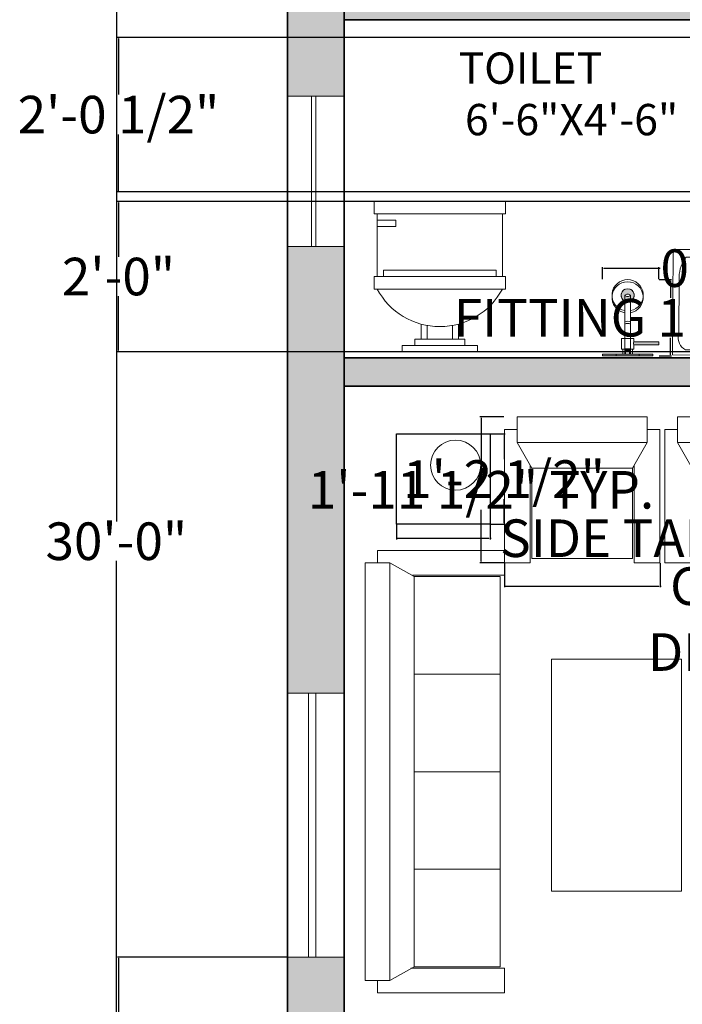
# Model space of a CAD drawing. Units: inches. Extents: x 143233372 to 143233714, y 112671713 to 112672292.
# Tile 2 of 7: x 143233373 to 143233479, y 112671935 to 112672092. Entities that reach past the tile are written whole.
import ezdxf

# ---------------------------------------------------------------- set-up
doc = ezdxf.new("R2010")
doc.units = ezdxf.units.IN
doc.header["$MEASUREMENT"] = 0
doc.layers.get('0').update_dxf_attribs({"color": 104})
for name, color, linetype, lineweight in [('A-ANNO-DIMS', 2, 'Continuous', 18), ('A-AREA-IDEN', 7, 'Continuous', 18), ('furniture', 23, 'Continuous', 18), ('PLUMBING FIXTURES', 8, 'Continuous', 18), ('walls', 7, 'Continuous', 35), ('windows', 4, 'Continuous', 18)]:
    doc.layers.add(name, color=color, linetype=linetype, lineweight=lineweight)
doc.layers.add('A-WALL-PATT', color=18, linetype='Continuous', lineweight=9, true_color=0x000000)
doc.layers.add('table', color=140, linetype='Continuous')
doc.styles.get("Standard").update_dxf_attribs({"font": 'arial.ttf'})
doc.dimstyles.get("Standard").update_dxf_attribs({"dimtxt": 6, "dimasz": 0.18, "dimexe": 0.18, "dimexo": 0.0625, "dimgap": 0.09, "dimtad": 0, "dimtih": 1, "dimtoh": 1, "dimzin": 0, "dimdsep": 46, "dimlunit": 3, "dimtxsty": 'Standard', "dimcen": 0.09, "dimadec": 0, "dimazin": 0, "dimtfac": 1, "dimtofl": 0, "dimtmove": 0, "dimatfit": 3, "dimfxl": 1, "dimtolj": 1, "dimtzin": 0, "dimarcsym": 0})

# ---------------------------------------------------------------- blocks, each defined once
blk = doc.blocks.new('FABRIC SOFA 4S')
at = {"layer": 'furniture'}
for p, q in [((3, 54), (34, 54)), ((3, 51), (3, 54)), ((34, 48), (34, 54)), ((0, -51), (0, 51)), ((6, 51), (0, 51)), ((6, -51), (6, 51)), ((12, 47.63), (6, 51)), ((11.14, 48), (34, 48)), ((33, 23.81), (12, 23.81)), ((33, 0), (12, 0)), ((33, -23.81), (12, -23.81)), ((6, -51), (12, -47.63)), ((11.54, -48), (34, -48)), ((34, -48), (34, -54)), ((6, -51), (0, -51)), ((3, -54), (3, -51)), ((3, -54), (34, -54))]:
    blk.add_line(p, q, dxfattribs=at)
blk.add_lwpolyline([(12, -47.63), (12, 47.63), (33, 47.63), (33, -47.63)], close=True, dxfattribs=at)
blk = doc.blocks.new('table')
at = {"layer": 'furniture'}
blk.add_circle((2425.82, 1326.97), 6.64, dxfattribs=at)
at = {"layer": 'table'}
blk.add_line((2410.17, 1335.23), (2434.94, 1335.23), dxfattribs=at)
blk = doc.blocks.new('support table')
at = {"layer": 'table'}
for p, q in [((-15.66, -15.62), (-15.66, 8.26)), ((9.12, 8.26), (9.12, -15.62)), ((9.12, -15.62), (-15.66, -15.62))]:
    blk.add_line(p, q, dxfattribs=at)
at = {"layer": 'furniture'}
blk.add_blockref('table', (-2425.82, -1326.97), dxfattribs=at)
blk = doc.blocks.new('FABRIC SOFA 1S')
at = {"layer": 'furniture'}
for p, q in [((3, 18.12), (34, 18.12)), ((3, 15.12), (3, 18.12)), ((34, 12.12), (34, 18.12)), ((0, -15.12), (0, 15.12)), ((6, 15.12), (0, 15.12)), ((6, -15.12), (6, 15.12)), ((12, 11.75), (6, 15.12)), ((11.33, 12.12), (34, 12.12)), ((6, -15.12), (12, -11.75)), ((11.33, -12.12), (34, -12.12)), ((34, -12.12), (34, -18.12)), ((6, -15.12), (0, -15.12)), ((3, -18.12), (3, -15.12)), ((3, -18.12), (34, -18.12))]:
    blk.add_line(p, q, dxfattribs=at)
blk.add_lwpolyline([(12, -11.75), (12, 11.75), (33, 11.75), (33, -11.75)], close=True, dxfattribs=at)
blk = doc.blocks.new('*U19')
for p, q in [((-10, 22), (-10, 12)), ((-10, 21), (-7, 21)), ((-7, 21), (-7, 20)), ((10, 12), (10, 22)), ((-7, 20), (-10, 20)), ((9, 13), (-9, 13)), ((-9, 13), (-9, 12)), ((9, 12), (9, 13)), ((10.5, 12), (-10.5, 12)), ((-10.5, 10), (-10.5, 12)), ((10.5, 12), (10.5, 10)), ((10.5, 10), (-10.5, 10)), ((-3, 4.4065), (-3, 2)), ((-2, 2), (-2, 4.1658)), ((2, 4.1658), (2, 2)), ((3, 2), (3, 4.4065)), ((4, 2), (-4, 2)), ((-4, 2), (-4, 1)), ((4, 1), (4, 2))]:
    blk.add_line(p, q)
for points in [[(10.5, 22), (10.5, 24), (-10.5, 24), (-10.5, 22)], [(6, 0), (6, 1), (-6, 1), (-6, 0)]]:
    blk.add_lwpolyline(points, close=True)
blk.add_arc((0, 15.3333), 11.3333, 208.0725, 331.9275)
blk = doc.blocks.new('O.H SHOWER-PL')
at = {"layer": 'PLUMBING FIXTURES'}
for points in [[(-1.84, 0), (-1.84, -0.25), (1.84, -0.25), (1.84, 0)], [(0.46, -8.72), (0.46, -9.67, -0.422337), (-0.46, -9.67), (-0.46, -8.72, 4.325472)]]:
    blk.add_hatch(color=256, dxfattribs=at).paths.add_polyline_path(points)
for p, q in [((-1.84, 0), (-1.84, -0.25)), ((1.84, 0), (-1.84, 0)), ((1.84, 0), (1.84, -0.25)), ((1.84, -0.25), (-1.84, -0.25)), ((-0.46, -0.25), (-0.46, -9.67)), ((0.46, -0.25), (0.46, -9.67))]:
    blk.add_line(p, q, dxfattribs=at)
for centre, radius, start, end in [((0, -4.48), 1.03, 243.53, 296.47), ((0, -9.67), 2.5, 100.61, 79.39), ((0, -9.67), 1.05, 116.0349, 63.9652), ((0, -9.22), 0.643, 224.2078, 315.7922)]:
    blk.add_arc(centre, radius, start, end, dxfattribs=at)
blk = doc.blocks.new('DIVERTER-PL')
at = {"layer": 'PLUMBING FIXTURES'}
for points in [[(4, 0), (-4, 0), (-4, -0.25), (4, -0.25)], [(0.38, -1.14), (0.38, -0.7), (-0.37, -0.7), (-0.37, -1.14)], [(1, -1.75, 0.30818), (1, -2.25), (5, -2.25), (5, -1.75)]]:
    blk.add_hatch(color=256, dxfattribs=at).paths.add_polyline_path(points)
for p, q in [((-4, 0), (-4, -0.25)), ((-4, 0), (4, 0)), ((4, 0), (4, -0.25)), ((-4, -0.25), (4, -0.25)), ((-4, -0.25), (4, -0.25)), ((-1, -1.05), (-0.37, -1.05)), ((-1, -1.05), (-1, -2.75)), ((-0.75, -0.25), (-0.75, -1.05)), ((-0.37, -0.7), (0.38, -0.7)), ((-0.37, -0.7), (-0.37, -1.14)), ((-0.37, -1.14), (0.38, -1.14)), ((-0.32, -0.7), (-0.32, -0.25)), ((0.32, -0.7), (0.32, -0.25)), ((0.38, -0.7), (0.38, -1.14)), ((0.38, -1.05), (1, -1.05)), ((0.75, -0.25), (0.75, -1.05)), ((1, -1.05), (1, -1.75)), ((-1, -2.75), (1, -2.75)), ((1, -2.25), (1, -2.75))]:
    blk.add_line(p, q, dxfattribs=at)
at = {"layer": 'PLUMBING FIXTURES', "ltscale": 12}
for p, q in [((1, -1.75), (5, -1.75)), ((1, -2.25), (5, -2.25)), ((5, -2.25), (5, -1.75))]:
    blk.add_line(p, q, dxfattribs=at)
at = {"layer": 'PLUMBING FIXTURES'}
blk.add_arc((1.37, -2), 0.444, 145.7435, 214.2565, dxfattribs=at)
blk = doc.blocks.new('A$C7F153053')
at = {"layer": 'PLUMBING FIXTURES', "xscale": -1, "rotation": 270}
for name in ['DIVERTER-PL', 'O.H SHOWER-PL']:
    blk.add_blockref(name, (12.17, 4), dxfattribs=at)
blk = doc.blocks.new('*D28')
at = {"layer": 'A-ANNO-DIMS', "color": 0, "lineweight": -2, "transparency": 16777216}
for p, q in [((143233416.22, 112672249.18), (143233388.75, 112672249.18)), ((143233388.93, 112672249), (143233388.93, 112672011.59)), ((143233388.93, 112671767.86), (143233388.93, 112672005.28)), ((143233416.22, 112671767.68), (143233388.75, 112671767.68))]:
    blk.add_line(p, q, dxfattribs=at)
at = {"layer": 'A-ANNO-DIMS', "color": 0, "transparency": 16777216}
for points in [[(143233388.9, 112672249), (143233388.96, 112672249), (143233388.93, 112672249.18)], [(143233388.9, 112671767.86), (143233388.96, 112671767.86), (143233388.93, 112671767.68)]]:
    blk.add_solid(points, dxfattribs=at)
at = {"layer": 'Defpoints', "color": 0, "transparency": 16777216}
for p in [(143233416.28, 112672249.18), (143233388.93, 112671767.68), (143233416.28, 112671767.68)]:
    blk.add_point(p, dxfattribs=at)
at = {"layer": 'A-ANNO-DIMS', "color": 0, "transparency": 16777216, "insert": (143233388.93, 112672008.43), "char_height": 6, "attachment_point": 5}
blk.add_mtext('\\A1;30\'-0"', dxfattribs=at)
blk = doc.blocks.new('SASH-42IN')
for p, q in [((0, 1.17), (42.12, 1.17)), ((42.12, 0), (0, 0)), ((42.12, 1.17), (42.12, 0))]:
    blk.add_line(p, q)
blk = doc.blocks.new('LAVATORY-RECT')
for p, q in [((0, 0.15), (0.11, 17)), ((0.11, 17), (23.11, 16.85)), ((20.97, 15.65), (2.15, 15.77)), ((23.11, 16.85), (23.1, 15.71)), ((23.1, 15.71), (23, 0)), ((0.99, 3.35), (1.05, 12.64)), ((21.96, 3.21), (22.03, 12.5)), ((11.22, 9.73), (11.16, 9.24)), ((11.36, 9.22), (11.4, 9.7)), ((10.4, 8.91), (9.84, 8.81)), ((10.52, 8.7), (9.87, 8.58)), ((11.84, 8.39), (12.22, 7.95)), ((11.97, 8.6), (12.36, 8.13)), ((23, 0), (0, 0.15)), ((21.95, 0.84), (2.06, 0.97))]:
    blk.add_line(p, q)
for radius in [2.61, 1.39, 0.816, 0.338]:
    blk.add_circle((11.22, 8.91), radius)
for centre, radius, start, end in [((6.46, 12.5), 5.4, 142.7525, 178.5493), ((16.62, 12.43), 5.4, 0.6949, 36.4918), ((3, 2.82), 2.08, 165.2338, 242.9258), ((12.7, 2.09), 9.33, 352.3124, 6.9318)]:
    blk.add_arc(centre, radius, start, end)
blk = doc.blocks.new('SHOWER-ARM-AND-HEAD')
blk.add_hatch(color=256).paths.add_polyline_path([(2.05, 10.36), (2.05, 9.42, 0.422337), (2.97, 9.42), (2.97, 10.36, -4.325472)])
blk.add_hatch(color=256).paths.add_polyline_path([(2.05, 10.36), (2.05, 9.42, 0.422337), (2.97, 9.42), (2.97, 10.36, -4.325472)])
blk.add_hatch(color=256).paths.add_polyline_path([(2.05, 10.36), (2.05, 9.42, 0.422337), (2.97, 9.42), (2.97, 10.36, -4.325472)])
blk.add_hatch(color=256).paths.add_polyline_path([(2.05, 10.36), (2.05, 9.42, 0.422337), (2.97, 9.42), (2.97, 10.36, -4.325472)])
blk.add_hatch(color=256).paths.add_polyline_path([(2.05, 10.36), (2.05, 9.42, 0.422337), (2.97, 9.42), (2.97, 10.36, -4.325472)])
blk.add_hatch(color=256).paths.add_polyline_path([(2.05, 10.36), (2.05, 9.42, 0.422337), (2.97, 9.42), (2.97, 10.36, -4.325472)])
blk.add_hatch(color=256).paths.add_polyline_path([(2.05, 10.36), (2.05, 9.42, 0.422337), (2.97, 9.42), (2.97, 10.36, -4.325472)])
blk.add_hatch(color=256).paths.add_polyline_path([(2.05, 10.36), (2.05, 9.42, 0.422337), (2.97, 9.42), (2.97, 10.36, -4.325472)])
blk.add_hatch(color=256).paths.add_polyline_path([(2.05, 10.36), (2.05, 9.42, 0.422337), (2.97, 9.42), (2.97, 10.36, -4.325472)])
blk.add_hatch(color=256).paths.add_polyline_path([(2.05, 10.36), (2.05, 9.42, 0.422337), (2.97, 9.42), (2.97, 10.36, -4.325472)])
blk.add_hatch(color=256).paths.add_polyline_path([(2.05, 10.36), (2.05, 9.42, 0.422337), (2.97, 9.42), (2.97, 10.36, -4.325472)])
blk.add_hatch(color=256).paths.add_polyline_path([(2.05, 10.36), (2.05, 9.42, 0.422337), (2.97, 9.42), (2.97, 10.36, -4.325472)])
blk.add_hatch(color=256).paths.add_polyline_path([(2.05, 10.36), (2.05, 9.42, 0.422337), (2.97, 9.42), (2.97, 10.36, -4.325472)])
blk.add_hatch(color=256).paths.add_polyline_path([(2.05, 10.36), (2.05, 9.42, 0.422337), (2.97, 9.42), (2.97, 10.36, -4.325472)])
blk.add_hatch(color=256).paths.add_polyline_path([(2.05, 10.36), (2.05, 9.42, 0.422337), (2.97, 9.42), (2.97, 10.36, -4.325472)])
blk.add_hatch(color=256).paths.add_polyline_path([(2.05, 10.36), (2.05, 9.42, 0.422337), (2.97, 9.42), (2.97, 10.36, -4.325472)])
blk.add_hatch(color=256).paths.add_polyline_path([(2.05, 10.36), (2.05, 9.42, 0.422337), (2.97, 9.42), (2.97, 10.36, -4.325472)])
blk.add_hatch(color=256).paths.add_polyline_path([(2.05, 10.36), (2.05, 9.42, 0.422337), (2.97, 9.42), (2.97, 10.36, -4.325472)])
blk.add_hatch(color=256).paths.add_polyline_path([(2.05, 10.36), (2.05, 9.42, 0.422337), (2.97, 9.42), (2.97, 10.36, -4.325472)])
blk.add_hatch(color=256).paths.add_polyline_path([(2.05, 10.36), (2.05, 9.42, 0.422337), (2.97, 9.42), (2.97, 10.36, -4.325472)])
blk.add_hatch(color=256).paths.add_polyline_path([(2.05, 10.36), (2.05, 9.42, 0.422337), (2.97, 9.42), (2.97, 10.36, -4.325472)])
blk.add_hatch(color=256).paths.add_polyline_path([(2.05, 10.36), (2.05, 9.42, 0.422337), (2.97, 9.42), (2.97, 10.36, -4.325472)])
blk.add_hatch(color=256).paths.add_polyline_path([(2.05, 10.36), (2.05, 9.42, 0.422337), (2.97, 9.42), (2.97, 10.36, -4.325472)])
blk.add_hatch(color=256).paths.add_polyline_path([(2.05, 10.36), (2.05, 9.42, 0.422337), (2.97, 9.42), (2.97, 10.36, -4.325472)])
blk.add_hatch(color=256).paths.add_polyline_path([(2.05, 10.36), (2.05, 9.42, 0.422337), (2.97, 9.42), (2.97, 10.36, -4.325472)])
blk.add_hatch(color=256).paths.add_polyline_path([(2.05, 10.36), (2.05, 9.42, 0.422337), (2.97, 9.42), (2.97, 10.36, -4.325472)])
blk.add_hatch(color=256).paths.add_polyline_path([(2.05, 10.36), (2.05, 9.42, 0.422337), (2.97, 9.42), (2.97, 10.36, -4.325472)])
blk.add_hatch(color=256).paths.add_polyline_path([(2.05, 10.36), (2.05, 9.42, 0.422337), (2.97, 9.42), (2.97, 10.36, -4.325472)])
blk.add_hatch(color=256).paths.add_polyline_path([(2.05, 10.36), (2.05, 9.42, 0.422337), (2.97, 9.42), (2.97, 10.36, -4.325472)])
blk.add_hatch(color=256).paths.add_polyline_path([(2.05, 10.36), (2.05, 9.42, 0.422337), (2.97, 9.42), (2.97, 10.36, -4.325472)])
blk.add_hatch(color=256).paths.add_polyline_path([(2.05, 10.36), (2.05, 9.42, 0.422337), (2.97, 9.42), (2.97, 10.36, -4.325472)])
blk.add_hatch(color=256).paths.add_polyline_path([(2.05, 10.36), (2.05, 9.42, 0.422337), (2.97, 9.42), (2.97, 10.36, -4.325472)])
blk.add_hatch(color=256).paths.add_polyline_path([(2.05, 10.36), (2.05, 9.42, 0.422337), (2.97, 9.42), (2.97, 10.36, -4.325472)])
blk.add_hatch(color=256).paths.add_polyline_path([(2.05, 10.36), (2.05, 9.42, 0.422337), (2.97, 9.42), (2.97, 10.36, -4.325472)])
blk.add_hatch(color=256).paths.add_polyline_path([(2.05, 10.36), (2.05, 9.42, 0.422337), (2.97, 9.42), (2.97, 10.36, -4.325472)])
blk.add_hatch(color=256).paths.add_polyline_path([(2.05, 10.36), (2.05, 9.42, 0.422337), (2.97, 9.42), (2.97, 10.36, -4.325472)])
blk.add_hatch(color=256).paths.add_polyline_path([(2.05, 10.36), (2.05, 9.42, 0.422337), (2.97, 9.42), (2.97, 10.36, -4.325472)])
blk.add_hatch(color=256).paths.add_polyline_path([(2.05, 10.36), (2.05, 9.42, 0.422337), (2.97, 9.42), (2.97, 10.36, -4.325472)])
for p, q in [((2.05, 0), (2.05, 9.42)), ((2.05, 0), (2.05, 9.42)), ((2.05, 0), (2.05, 9.42)), ((2.05, 0), (2.05, 9.42)), ((2.05, 0), (2.05, 9.42)), ((2.05, 0), (2.05, 9.42)), ((2.05, 0), (2.05, 9.42)), ((2.05, 0), (2.05, 9.42)), ((2.05, 0), (2.05, 9.42)), ((2.05, 0), (2.05, 9.42)), ((2.05, 0), (2.05, 9.42)), ((2.05, 0), (2.05, 9.42)), ((2.05, 0), (2.05, 9.42)), ((2.05, 0), (2.05, 9.42)), ((2.05, 0), (2.05, 9.42)), ((2.05, 0), (2.05, 9.42)), ((2.05, 0), (2.05, 9.42)), ((2.05, 0), (2.05, 9.42)), ((2.05, 0), (2.05, 9.42)), ((2.05, 0), (2.05, 9.42)), ((2.05, 0), (2.05, 9.42)), ((2.05, 0), (2.05, 9.42)), ((2.05, 0), (2.05, 9.42)), ((2.05, 0), (2.05, 9.42)), ((2.05, 0), (2.05, 9.42)), ((2.05, 0), (2.05, 9.42)), ((2.05, 0), (2.05, 9.42)), ((2.05, 0), (2.05, 9.42)), ((2.05, 0), (2.05, 9.42)), ((2.05, 0), (2.05, 9.42)), ((2.05, 0), (2.05, 9.42)), ((2.05, 0), (2.05, 9.42)), ((2.05, 0), (2.05, 9.42)), ((2.05, 0), (2.05, 9.42)), ((2.05, 0), (2.05, 9.42)), ((2.05, 0), (2.05, 9.42)), ((2.05, 0), (2.05, 9.42)), ((2.05, 0), (2.05, 9.42)), ((2.97, 0), (2.97, 9.42)), ((2.97, 0), (2.97, 9.42)), ((2.97, 0), (2.97, 9.42)), ((2.97, 0), (2.97, 9.42)), ((2.97, 0), (2.97, 9.42)), ((2.97, 0), (2.97, 9.42)), ((2.97, 0), (2.97, 9.42)), ((2.97, 0), (2.97, 9.42)), ((2.97, 0), (2.97, 9.42)), ((2.97, 0), (2.97, 9.42)), ((2.97, 0), (2.97, 9.42)), ((2.97, 0), (2.97, 9.42)), ((2.97, 0), (2.97, 9.42)), ((2.97, 0), (2.97, 9.42)), ((2.97, 0), (2.97, 9.42)), ((2.97, 0), (2.97, 9.42)), ((2.97, 0), (2.97, 9.42)), ((2.97, 0), (2.97, 9.42)), ((2.97, 0), (2.97, 9.42)), ((2.97, 0), (2.97, 9.42)), ((2.97, 0), (2.97, 9.42)), ((2.97, 0), (2.97, 9.42)), ((2.97, 0), (2.97, 9.42)), ((2.97, 0), (2.97, 9.42)), ((2.97, 0), (2.97, 9.42)), ((2.97, 0), (2.97, 9.42)), ((2.97, 0), (2.97, 9.42)), ((2.97, 0), (2.97, 9.42)), ((2.97, 0), (2.97, 9.42)), ((2.97, 0), (2.97, 9.42)), ((2.97, 0), (2.97, 9.42)), ((2.97, 0), (2.97, 9.42)), ((2.97, 0), (2.97, 9.42)), ((2.97, 0), (2.97, 9.42)), ((2.97, 0), (2.97, 9.42)), ((2.97, 0), (2.97, 9.42)), ((2.97, 0), (2.97, 9.42)), ((2.97, 0), (2.97, 9.42))]:
    blk.add_line(p, q)
for centre, radius, start, end in [((2.5, 9.07), 2.5, 280.61, 259.39), ((2.5, 9.07), 2.5, 280.61, 259.39), ((2.5, 9.07), 2.5, 280.61, 259.39), ((2.5, 9.07), 2.5, 280.61, 259.39), ((2.5, 9.07), 2.5, 280.61, 259.39), ((2.5, 9.07), 2.5, 280.61, 259.39), ((2.5, 9.07), 2.5, 280.61, 259.39), ((2.5, 9.07), 2.5, 280.61, 259.39), ((2.5, 9.07), 2.5, 280.61, 259.39), ((2.5, 9.07), 2.5, 280.61, 259.39), ((2.5, 9.07), 2.5, 280.61, 259.39), ((2.5, 9.07), 2.5, 280.61, 259.39), ((2.5, 9.07), 2.5, 280.61, 259.39), ((2.5, 9.07), 2.5, 280.61, 259.39), ((2.5, 9.07), 2.5, 280.61, 259.39), ((2.5, 9.07), 2.5, 280.61, 259.39), ((2.5, 9.07), 2.5, 280.61, 259.39), ((2.5, 9.07), 2.5, 280.61, 259.39), ((2.5, 9.07), 2.5, 280.61, 259.39), ((2.5, 9.07), 2.5, 280.61, 259.39), ((2.5, 9.07), 2.5, 280.61, 259.39), ((2.5, 9.07), 2.5, 280.61, 259.39), ((2.5, 9.07), 2.5, 280.61, 259.39), ((2.5, 9.07), 2.5, 280.61, 259.39), ((2.5, 9.07), 2.5, 280.61, 259.39), ((2.5, 9.07), 2.5, 280.61, 259.39), ((2.5, 9.07), 2.5, 280.61, 259.39), ((2.5, 9.07), 2.5, 280.61, 259.39), ((2.5, 9.07), 2.5, 280.61, 259.39), ((2.5, 9.07), 2.5, 280.61, 259.39), ((2.5, 9.07), 2.5, 280.61, 259.39), ((2.5, 9.07), 2.5, 280.61, 259.39), ((2.5, 9.07), 2.5, 280.61, 259.39), ((2.5, 9.07), 2.5, 280.61, 259.39), ((2.5, 9.07), 2.5, 280.61, 259.39), ((2.5, 9.07), 2.5, 280.61, 259.39), ((2.5, 9.07), 2.5, 280.61, 259.39), ((2.5, 9.07), 2.5, 280.61, 259.39), ((2.51, 9.42), 1.05, 116.0348, 63.9651), ((2.51, 9.42), 1.05, 116.0348, 63.9651), ((2.51, 9.42), 1.05, 116.0348, 63.9651), ((2.51, 9.42), 1.05, 116.0348, 63.9651), ((2.51, 9.42), 1.05, 116.0348, 63.9651), ((2.51, 9.42), 1.05, 116.0348, 63.9651), ((2.51, 9.42), 1.05, 116.0348, 63.9651), ((2.51, 9.42), 1.05, 116.0348, 63.9651), ((2.51, 9.42), 1.05, 116.0348, 63.9651), ((2.51, 9.42), 1.05, 116.0348, 63.9651), ((2.51, 9.42), 1.05, 116.0348, 63.9651), ((2.51, 9.42), 1.05, 116.0348, 63.9651), ((2.51, 9.42), 1.05, 116.0348, 63.9651), ((2.51, 9.42), 1.05, 116.0348, 63.9651), ((2.51, 9.42), 1.05, 116.0348, 63.9651), ((2.51, 9.42), 1.05, 116.0348, 63.9651), ((2.51, 9.42), 1.05, 116.0348, 63.9651), ((2.51, 9.42), 1.05, 116.0348, 63.9651), ((2.51, 9.42), 1.05, 116.0348, 63.9651), ((2.51, 9.42), 1.05, 116.0348, 63.9651), ((2.51, 9.42), 1.05, 116.0348, 63.9651), ((2.51, 9.42), 1.05, 116.0348, 63.9651), ((2.51, 9.42), 1.05, 116.0348, 63.9651), ((2.51, 9.42), 1.05, 116.0348, 63.9651), ((2.51, 9.42), 1.05, 116.0348, 63.9651), ((2.51, 9.42), 1.05, 116.0348, 63.9651), ((2.51, 9.42), 1.05, 116.0348, 63.9651), ((2.51, 9.42), 1.05, 116.0348, 63.9651), ((2.51, 9.42), 1.05, 116.0348, 63.9651), ((2.51, 9.42), 1.05, 116.0348, 63.9651), ((2.51, 9.42), 1.05, 116.0348, 63.9651), ((2.51, 9.42), 1.05, 116.0348, 63.9651), ((2.51, 9.42), 1.05, 116.0348, 63.9651), ((2.51, 9.42), 1.05, 116.0348, 63.9651), ((2.51, 9.42), 1.05, 116.0348, 63.9651), ((2.51, 9.42), 1.05, 116.0348, 63.9651), ((2.51, 9.42), 1.05, 116.0348, 63.9651), ((2.51, 9.42), 1.05, 116.0348, 63.9651), ((2.51, 9.87), 0.643, 224.2078, 315.7922), ((2.51, 9.87), 0.643, 224.2078, 315.7922), ((2.51, 9.87), 0.643, 224.2078, 315.7922), ((2.51, 9.87), 0.643, 224.2078, 315.7922), ((2.51, 9.87), 0.643, 224.2078, 315.7922), ((2.51, 9.87), 0.643, 224.2078, 315.7922), ((2.51, 9.87), 0.643, 224.2078, 315.7922), ((2.51, 9.87), 0.643, 224.2078, 315.7922), ((2.51, 9.87), 0.643, 224.2078, 315.7922), ((2.51, 9.87), 0.643, 224.2078, 315.7922), ((2.51, 9.87), 0.643, 224.2078, 315.7922), ((2.51, 9.87), 0.643, 224.2078, 315.7922), ((2.51, 9.87), 0.643, 224.2078, 315.7922), ((2.51, 9.87), 0.643, 224.2078, 315.7922), ((2.51, 9.87), 0.643, 224.2078, 315.7922), ((2.51, 9.87), 0.643, 224.2078, 315.7922), ((2.51, 9.87), 0.643, 224.2078, 315.7922), ((2.51, 9.87), 0.643, 224.2078, 315.7922), ((2.51, 9.87), 0.643, 224.2078, 315.7922), ((2.51, 9.87), 0.643, 224.2078, 315.7922), ((2.51, 9.87), 0.643, 224.2078, 315.7922), ((2.51, 9.87), 0.643, 224.2078, 315.7922), ((2.51, 9.87), 0.643, 224.2078, 315.7922), ((2.51, 9.87), 0.643, 224.2078, 315.7922), ((2.51, 9.87), 0.643, 224.2078, 315.7922), ((2.51, 9.87), 0.643, 224.2078, 315.7922), ((2.51, 9.87), 0.643, 224.2078, 315.7922), ((2.51, 9.87), 0.643, 224.2078, 315.7922), ((2.51, 9.87), 0.643, 224.2078, 315.7922), ((2.51, 9.87), 0.643, 224.2078, 315.7922), ((2.51, 9.87), 0.643, 224.2078, 315.7922), ((2.51, 9.87), 0.643, 224.2078, 315.7922), ((2.51, 9.87), 0.643, 224.2078, 315.7922), ((2.51, 9.87), 0.643, 224.2078, 315.7922), ((2.51, 9.87), 0.643, 224.2078, 315.7922), ((2.51, 9.87), 0.643, 224.2078, 315.7922), ((2.51, 9.87), 0.643, 224.2078, 315.7922), ((2.51, 9.87), 0.643, 224.2078, 315.7922), ((2.5, 3.88), 1.03, 63.53, 116.47), ((2.5, 3.88), 1.03, 63.53, 116.47), ((2.5, 3.88), 1.03, 63.53, 116.47), ((2.5, 3.88), 1.03, 63.53, 116.47), ((2.5, 3.88), 1.03, 63.53, 116.47), ((2.5, 3.88), 1.03, 63.53, 116.47), ((2.5, 3.88), 1.03, 63.53, 116.47), ((2.5, 3.88), 1.03, 63.53, 116.47), ((2.5, 3.88), 1.03, 63.53, 116.47), ((2.5, 3.88), 1.03, 63.53, 116.47), ((2.5, 3.88), 1.03, 63.53, 116.47), ((2.5, 3.88), 1.03, 63.53, 116.47), ((2.5, 3.88), 1.03, 63.53, 116.47), ((2.5, 3.88), 1.03, 63.53, 116.47), ((2.5, 3.88), 1.03, 63.53, 116.47), ((2.5, 3.88), 1.03, 63.53, 116.47), ((2.5, 3.88), 1.03, 63.53, 116.47), ((2.5, 3.88), 1.03, 63.53, 116.47), ((2.5, 3.88), 1.03, 63.53, 116.47), ((2.5, 3.88), 1.03, 63.53, 116.47), ((2.5, 3.88), 1.03, 63.53, 116.47), ((2.5, 3.88), 1.03, 63.53, 116.47), ((2.5, 3.88), 1.03, 63.53, 116.47), ((2.5, 3.88), 1.03, 63.53, 116.47), ((2.5, 3.88), 1.03, 63.53, 116.47), ((2.5, 3.88), 1.03, 63.53, 116.47), ((2.5, 3.88), 1.03, 63.53, 116.47), ((2.5, 3.88), 1.03, 63.53, 116.47), ((2.5, 3.88), 1.03, 63.53, 116.47), ((2.5, 3.88), 1.03, 63.53, 116.47), ((2.5, 3.88), 1.03, 63.53, 116.47), ((2.5, 3.88), 1.03, 63.53, 116.47), ((2.5, 3.88), 1.03, 63.53, 116.47), ((2.5, 3.88), 1.03, 63.53, 116.47), ((2.5, 3.88), 1.03, 63.53, 116.47), ((2.5, 3.88), 1.03, 63.53, 116.47), ((2.5, 3.88), 1.03, 63.53, 116.47), ((2.5, 3.88), 1.03, 63.53, 116.47)]:
    blk.add_arc(centre, radius, start, end)
blk = doc.blocks.new('*D35')
at = {"layer": 'A-ANNO-DIMS', "color": 0, "lineweight": -2, "transparency": 16777216}
for p, q in [((143233450.89, 112672004.93), (143233450.89, 112672001.08)), ((143233475.74, 112672004.93), (143233475.74, 112672001.08)), ((143233451.07, 112672001.26), (143233475.56, 112672001.26)), ((143233475.74, 112672001.26), (143233475.92, 112672001.26))]:
    blk.add_line(p, q, dxfattribs=at)
at = {"layer": 'A-ANNO-DIMS', "color": 0, "transparency": 16777216}
for points in [[(143233451.07, 112672001.29), (143233451.07, 112672001.23), (143233450.89, 112672001.26)], [(143233475.56, 112672001.29), (143233475.56, 112672001.23), (143233475.74, 112672001.26)]]:
    blk.add_solid(points, dxfattribs=at)
at = {"layer": 'Defpoints', "color": 0, "transparency": 16777216}
for p in [(143233450.89, 112672004.99), (143233475.74, 112672004.99), (143233475.74, 112672001.26)]:
    blk.add_point(p, dxfattribs=at)
at = {"layer": 'A-ANNO-DIMS', "color": 0, "transparency": 16777216, "insert": (143233508.46, 112672001.26), "char_height": 6, "attachment_point": 5}
blk.add_mtext('\\A1;CHAIR 2\'-1" TYP.', dxfattribs=at)
blk = doc.blocks.new('*D36')
at = {"layer": 'A-ANNO-DIMS', "color": 0, "lineweight": -2, "transparency": 16777216}
for p, q in [((143233450.82, 112672028.3), (143233446.98, 112672028.3)), ((143233447.16, 112672028.12), (143233447.16, 112672019.84)), ((143233447.16, 112672005.17), (143233447.16, 112672013.45)), ((143233450.82, 112672004.99), (143233446.98, 112672004.99))]:
    blk.add_line(p, q, dxfattribs=at)
at = {"layer": 'A-ANNO-DIMS', "color": 0, "transparency": 16777216}
for points in [[(143233447.13, 112672028.12), (143233447.19, 112672028.12), (143233447.16, 112672028.3)], [(143233447.13, 112672005.17), (143233447.19, 112672005.17), (143233447.16, 112672004.99)]]:
    blk.add_solid(points, dxfattribs=at)
at = {"layer": 'Defpoints', "color": 0, "transparency": 16777216}
for p in [(143233450.89, 112672028.3), (143233447.16, 112672004.99), (143233450.89, 112672004.99)]:
    blk.add_point(p, dxfattribs=at)
at = {"layer": 'A-ANNO-DIMS', "color": 0, "transparency": 16777216, "insert": (143233447.16, 112672016.64), "char_height": 6, "attachment_point": 5}
blk.add_mtext('\\A1;1\'-11 1/2" TYP.', dxfattribs=at)
blk = doc.blocks.new('*D49')
at = {"layer": 'A-ANNO-DIMS', "color": 0, "lineweight": -2, "transparency": 16777216}
for p, q in [((143233475.63, 112672050.2), (143233477.58, 112672050.2)), ((143233477.4, 112672050.02), (143233477.4, 112672047.31)), ((143233477.4, 112672038.21), (143233477.4, 112672040.92)), ((143233475.63, 112672038.03), (143233477.58, 112672038.03))]:
    blk.add_line(p, q, dxfattribs=at)
at = {"layer": 'A-ANNO-DIMS', "color": 0, "transparency": 16777216}
for points in [[(143233477.37, 112672050.02), (143233477.43, 112672050.02), (143233477.4, 112672050.2)], [(143233477.37, 112672038.21), (143233477.43, 112672038.21), (143233477.4, 112672038.03)]]:
    blk.add_solid(points, dxfattribs=at)
at = {"layer": 'Defpoints', "color": 0, "transparency": 16777216}
for p in [(143233475.57, 112672050.2), (143233475.57, 112672038.03), (143233477.4, 112672038.03)]:
    blk.add_point(p, dxfattribs=at)
at = {"layer": 'A-ANNO-DIMS', "color": 0, "transparency": 16777216, "insert": (143233477.4, 112672044.11), "char_height": 6, "attachment_point": 5}
blk.add_mtext('\\A1;FITTING 1\'-0" TYP.', dxfattribs=at)
blk = doc.blocks.new('*D50')
at = {"layer": 'A-ANNO-DIMS', "color": 0, "lineweight": -2, "transparency": 16777216}
for p, q in [((143233466.57, 112672050.26), (143233466.57, 112672052.2)), ((143233466.75, 112672052.02), (143233475.39, 112672052.02)), ((143233475.57, 112672050.26), (143233475.57, 112672052.2)), ((143233475.57, 112672052.02), (143233475.75, 112672052.02))]:
    blk.add_line(p, q, dxfattribs=at)
at = {"layer": 'A-ANNO-DIMS', "color": 0, "transparency": 16777216}
for points in [[(143233466.75, 112672052.05), (143233466.75, 112672051.99), (143233466.57, 112672052.02)], [(143233475.39, 112672052.05), (143233475.39, 112672051.99), (143233475.57, 112672052.02)]]:
    blk.add_solid(points, dxfattribs=at)
at = {"layer": 'Defpoints', "color": 0, "transparency": 16777216}
for p in [(143233475.57, 112672052.02), (143233466.57, 112672050.2), (143233475.57, 112672050.2)]:
    blk.add_point(p, dxfattribs=at)
at = {"layer": 'A-ANNO-DIMS', "color": 0, "transparency": 16777216, "insert": (143233494.13, 112672052.02), "char_height": 6, "attachment_point": 5}
blk.add_mtext('\\A1;0\'-9" TYP.', dxfattribs=at)
blk = doc.blocks.new('*D55')
at = {"layer": 'A-ANNO-DIMS', "color": 0, "lineweight": -2, "transparency": 16777216}
for p, q in [((143233433.65, 112672011.09), (143233433.65, 112672008.73)), ((143233448.6, 112672011.09), (143233448.6, 112672008.73)), ((143233433.83, 112672008.91), (143233448.42, 112672008.91)), ((143233448.6, 112672008.91), (143233448.78, 112672008.91))]:
    blk.add_line(p, q, dxfattribs=at)
at = {"layer": 'A-ANNO-DIMS', "color": 0, "transparency": 16777216}
for points in [[(143233433.83, 112672008.94), (143233433.83, 112672008.88), (143233433.65, 112672008.91)], [(143233448.42, 112672008.94), (143233448.42, 112672008.88), (143233448.6, 112672008.91)]]:
    blk.add_solid(points, dxfattribs=at)
at = {"layer": 'Defpoints', "color": 0, "transparency": 16777216}
for p in [(143233433.65, 112672011.15), (143233448.6, 112672011.15), (143233448.6, 112672008.91)]:
    blk.add_point(p, dxfattribs=at)
at = {"layer": 'A-ANNO-DIMS', "color": 0, "transparency": 16777216, "insert": (143233482.22, 112672008.91), "char_height": 6, "attachment_point": 5}
blk.add_mtext('\\A1;SIDE TABLE 1\'-3"', dxfattribs=at)
blk = doc.blocks.new('*D56')
at = {"layer": 'A-ANNO-DIMS', "color": 0, "lineweight": -2, "transparency": 16777216}
for p, q in [((143233448.66, 112672025.56), (143233451.02, 112672025.56)), ((143233450.84, 112672025.38), (143233450.84, 112672021.55)), ((143233450.84, 112672011.33), (143233450.84, 112672015.16)), ((143233448.66, 112672011.15), (143233451.02, 112672011.15))]:
    blk.add_line(p, q, dxfattribs=at)
at = {"layer": 'A-ANNO-DIMS', "color": 0, "transparency": 16777216}
for points in [[(143233450.81, 112672025.38), (143233450.87, 112672025.38), (143233450.84, 112672025.56)], [(143233450.81, 112672011.33), (143233450.87, 112672011.33), (143233450.84, 112672011.15)]]:
    blk.add_solid(points, dxfattribs=at)
at = {"layer": 'Defpoints', "color": 0, "transparency": 16777216}
for p in [(143233448.6, 112672025.56), (143233450.84, 112672025.56), (143233448.6, 112672011.15)]:
    blk.add_point(p, dxfattribs=at)
at = {"layer": 'A-ANNO-DIMS', "color": 0, "transparency": 16777216, "insert": (143233450.84, 112672018.35), "char_height": 6, "attachment_point": 5}
blk.add_mtext('\\A1;1\'-2 1/2"', dxfattribs=at)
blk = doc.blocks.new('*D61')
at = {"layer": 'A-ANNO-DIMS', "color": 0, "lineweight": -2, "transparency": 16777216}
for p, q in [((143233522.04, 112672021.05), (143233512.83, 112672021.05)), ((143233513.01, 112672020.87), (143233513.01, 112671993.94)), ((143233513.01, 112671960.62), (143233513.01, 112671987.55)), ((143233522.04, 112671960.44), (143233512.83, 112671960.44))]:
    blk.add_line(p, q, dxfattribs=at)
at = {"layer": 'A-ANNO-DIMS', "color": 0, "transparency": 16777216}
for points in [[(143233512.98, 112672020.87), (143233513.04, 112672020.87), (143233513.01, 112672021.05)], [(143233512.98, 112671960.62), (143233513.04, 112671960.62), (143233513.01, 112671960.44)]]:
    blk.add_solid(points, dxfattribs=at)
at = {"layer": 'Defpoints', "color": 0, "transparency": 16777216}
for p in [(143233513.01, 112672021.05), (143233522.1, 112672021.05), (143233522.1, 112671960.44)]:
    blk.add_point(p, dxfattribs=at)
at = {"layer": 'A-ANNO-DIMS', "color": 0, "transparency": 16777216, "insert": (143233513.01, 112671990.74), "char_height": 6, "attachment_point": 5}
blk.add_mtext('\\A1;DINING SET 5\'-0 1/2"', dxfattribs=at)
blk = doc.blocks.new('*D70')
at = {"layer": 'A-ANNO-DIMS', "color": 0, "lineweight": -2, "transparency": 16777216}
for p, q in [((143233574.42, 112672088.85), (143233389.09, 112672088.85)), ((143233389.27, 112672088.67), (143233389.27, 112672079.72)), ((143233389.27, 112672064.38), (143233389.27, 112672073.33)), ((143233575.22, 112672064.2), (143233389.09, 112672064.2))]:
    blk.add_line(p, q, dxfattribs=at)
at = {"layer": 'A-ANNO-DIMS', "color": 0, "transparency": 16777216}
for points in [[(143233389.24, 112672088.67), (143233389.3, 112672088.67), (143233389.27, 112672088.85)], [(143233389.24, 112672064.38), (143233389.3, 112672064.38), (143233389.27, 112672064.2)]]:
    blk.add_solid(points, dxfattribs=at)
at = {"layer": 'Defpoints', "color": 0, "transparency": 16777216}
for p in [(143233574.48, 112672088.85), (143233389.27, 112672064.2), (143233575.28, 112672064.2)]:
    blk.add_point(p, dxfattribs=at)
at = {"layer": 'A-ANNO-DIMS', "color": 0, "transparency": 16777216, "insert": (143233389.27, 112672076.53), "char_height": 6, "attachment_point": 5}
blk.add_mtext('\\A1;2\'-0 1/2"', dxfattribs=at)
blk = doc.blocks.new('*D72')
at = {"layer": 'A-ANNO-DIMS', "color": 0, "lineweight": -2, "transparency": 16777216}
for p, q in [((143233576.46, 112672062.68), (143233389.09, 112672062.68)), ((143233389.27, 112672062.5), (143233389.27, 112672053.84)), ((143233389.27, 112672038.86), (143233389.27, 112672047.53)), ((143233586.96, 112672038.68), (143233389.09, 112672038.68))]:
    blk.add_line(p, q, dxfattribs=at)
at = {"layer": 'A-ANNO-DIMS', "color": 0, "transparency": 16777216}
for points in [[(143233389.24, 112672062.5), (143233389.3, 112672062.5), (143233389.27, 112672062.68)], [(143233389.24, 112672038.86), (143233389.3, 112672038.86), (143233389.27, 112672038.68)]]:
    blk.add_solid(points, dxfattribs=at)
at = {"layer": 'Defpoints', "color": 0, "transparency": 16777216}
for p in [(143233576.53, 112672062.68), (143233389.27, 112672038.68), (143233587.03, 112672038.68)]:
    blk.add_point(p, dxfattribs=at)
at = {"layer": 'A-ANNO-DIMS', "color": 0, "transparency": 16777216, "insert": (143233389.27, 112672050.68), "char_height": 6, "attachment_point": 5}
blk.add_mtext('\\A1;2\'-0"', dxfattribs=at)
blk = doc.blocks.new('*D73')
at = {"layer": 'A-ANNO-DIMS', "color": 0, "lineweight": -2, "transparency": 16777216}
for p, q in [((143233416.22, 112671942.04), (143233389.09, 112671942.04)), ((143233389.27, 112671941.86), (143233389.27, 112671905.44)), ((143233389.27, 112671862.63), (143233389.27, 112671899.05)), ((143233416.22, 112671862.45), (143233389.09, 112671862.45))]:
    blk.add_line(p, q, dxfattribs=at)
at = {"layer": 'A-ANNO-DIMS', "color": 0, "transparency": 16777216}
for points in [[(143233389.24, 112671941.86), (143233389.3, 112671941.86), (143233389.27, 112671942.04)], [(143233389.24, 112671862.63), (143233389.3, 112671862.63), (143233389.27, 112671862.45)]]:
    blk.add_solid(points, dxfattribs=at)
at = {"layer": 'Defpoints', "color": 0, "transparency": 16777216}
for p in [(143233389.27, 112671942.04), (143233416.28, 112671942.04), (143233416.28, 112671862.45)]:
    blk.add_point(p, dxfattribs=at)
at = {"layer": 'A-ANNO-DIMS', "color": 0, "transparency": 16777216, "insert": (143233389.27, 112671902.24), "char_height": 6, "attachment_point": 5}
blk.add_mtext('\\A1;6\'-7 1/2"', dxfattribs=at)

msp = doc.modelspace()

# ---------------------------------------------------------------- hatches: boundary and pattern name
at = {"layer": 'A-WALL-PATT'}
h = msp.add_hatch(color=256, dxfattribs=at)
h.dxf.hatch_style = 1
h.paths.add_polyline_path([(143233425.285, 112671820.328), (143233416.222, 112671820.328), (143233416.222, 112671767.682), (143233464.805, 112671767.682), (143233464.805, 112671776.682), (143233425.285, 112671776.682)])
h.paths.add_polyline_path([(143233425.285, 112672055.48), (143233416.285, 112672055.48), (143233416.285, 112671984.159), (143233425.285, 112671984.159)])
h.paths.add_polyline_path([(143233656.285, 112671963.912), (143233647.285, 112671963.912), (143233647.285, 112671848.682), (143233647.285, 112671839.682), (143233656.285, 112671839.682), (143233656.285, 112671889.182)])
h.paths.add_polyline_path([(143233425.285, 112672097.332), (143233425.285, 112672097.332), (143233425.285, 112672108.216), (143233425.285, 112672240.182), (143233451.497, 112672240.182), (143233451.497, 112672249.182), (143233416.285, 112672249.182), (143233416.285, 112672079.453), (143233420.069, 112672079.453), (143233425.285, 112672079.453)])
h.paths.add_polyline_path([(143233576.214, 112672249.182), (143233493.616, 112672249.182), (143233493.616, 112672240.182), (143233576.214, 112672240.182)])
h.paths.add_polyline_path([(143233425.285, 112671942.039), (143233416.285, 112671942.039), (143233416.285, 112671889.182), (143233416.271, 112671862.447), (143233425.285, 112671862.447), (143233425.285, 112671896.682), (143233518.63, 112671896.682, -0.0122006), (143233518.603, 112671897.787), (143233518.603, 112671901.182), (143233425.285, 112671901.182)])
h = msp.add_hatch(color=256, dxfattribs=at)
h.dxf.hatch_style = 1
h.paths.add_polyline_path([(143233507.785, 112672062.229), (143233504.087, 112672062.229, -0.0081431), (143233503.285, 112672062.242), (143233503.285, 112672037.682), (143233425.285, 112672037.682), (143233425.285, 112672033.182), (143233507.785, 112672033.182)])
h.paths.add_polyline_path([(143233511.719, 112672096.182), (143233425.285, 112672096.182), (143233425.285, 112672091.682), (143233503.285, 112672091.682), (143233503.285, 112672086.878), (143233504.087, 112672086.878), (143233507.785, 112672086.878), (143233507.785, 112672091.682), (143233511.719, 112672091.682)])

# ---------------------------------------------------------------- linework, layer by layer
at = {"layer": 'furniture'}
for p, q in [((143233433.654, 112672025.56), (143233433.654, 112672011.149)), ((143233448.599, 112672025.56), (143233433.654, 112672025.56)), ((143233448.599, 112672011.149), (143233448.599, 112672025.56)), ((143233433.654, 112672011.149), (143233448.599, 112672011.149)), ((143233458.405, 112671989.621), (143233458.405, 112671952.591)), ((143233479.165, 112671989.621), (143233458.405, 112671989.621)), ((143233479.165, 112671952.591), (143233479.165, 112671989.621)), ((143233458.405, 112671952.591), (143233479.165, 112671952.591))]:
    msp.add_line(p, q, dxfattribs=at)
at = {"layer": 'walls'}
for p, q in [((143233416.285, 112671889.182), (143233416.285, 112672249.182)), ((143233425.285, 112671901.182), (143233425.285, 112672240.182)), ((143233425.285, 112672091.682), (143233503.285, 112672091.682)), ((143233425.285, 112672037.682), (143233503.285, 112672037.682)), ((143233425.285, 112672033.182), (143233507.785, 112672033.182))]:
    msp.add_line(p, q, dxfattribs=at)
at = {"layer": 'windows'}
for p, q in [((143233416.285, 112672079.453), (143233425.285, 112672079.453)), ((143233416.285, 112672079.453), (143233420.069, 112672079.453)), ((143233420.069, 112672079.453), (143233420.069, 112672055.48)), ((143233420.785, 112672055.48), (143233420.785, 112672079.453)), ((143233425.285, 112672055.48), (143233416.285, 112672055.48)), ((143233420.069, 112672055.48), (143233420.785, 112672055.48)), ((143233425.285, 112671984.159), (143233416.285, 112671984.159)), ((143233416.285, 112671942.039), (143233425.285, 112671942.039))]:
    msp.add_line(p, q, dxfattribs=at)

# ---------------------------------------------------------------- block references
at = {"layer": 'furniture'}
for name, p, xscale, yscale, zscale, rotation in [('FABRIC SOFA 1S', (143233463.312, 112672028.298), 0.685544738852578, 0.685544738852578, 0.685544738852578, 270), ('FABRIC SOFA 1S', (143233488.92, 112672028.298), 0.685544738852578, 0.685544738852578, 0.685544738852578, 270), ('FABRIC SOFA 4S', (143233428.658, 112671971.646), -0.6537939928824033, 0.6537939928824033, 0.6537939928824033, 179.9999999998931)]:
    msp.add_blockref(name, p, dxfattribs=dict(at, xscale=xscale, yscale=yscale, zscale=zscale, rotation=rotation))
at = {"layer": 'furniture', "xscale": 0.6032856936233855, "yscale": 0.6032856936233855, "zscale": 0.6032856936233855}
msp.add_blockref('support table', (143233443.098, 112672020.575), dxfattribs=at)
at = {"layer": 'PLUMBING FIXTURES'}
for name, p in [('*U19', (143233440.58, 112672038.682)), ('LAVATORY-RECT', (143233477.735, 112672038.024)), ('SHOWER-ARM-AND-HEAD', (143233468.064, 112672038.279))]:
    msp.add_blockref(name, p, dxfattribs=at)
at = {"layer": 'PLUMBING FIXTURES', "ltscale": 35, "rotation": 270}
msp.add_blockref('A$C7F153053', (143233466.571, 112672050.195), dxfattribs=at)
at = {"layer": 'windows', "rotation": 90.00000009054449}
msp.add_blockref('SASH-42IN', (143233420.785, 112671942.04), dxfattribs=at)

# ---------------------------------------------------------------- texts
at = {"layer": 'A-AREA-IDEN'}
for s, p in [('TOILET', (143233443.581, 112672081.447)), ('6\'-6"X4\'-6"', (143233444.599, 112672073.233))]:
    msp.add_text(s, height=5, dxfattribs=at).set_placement(p)

# ---------------------------------------------------------------- dimensions: what is measured, and where the dimension line sits
at = {"layer": 'A-ANNO-DIMS'}
for base, p1, p2, angle, text, override, picture, middle in [((143233388.932, 112671767.682), (143233416.285, 112672249.182), (143233416.285, 112671767.682), 90, '30\'-0"', {"dimclrd": 0, "dimclre": 0, "dimclrt": 0}, '*D28', (143233388.932, 112672008.432)), ((143233477.396, 112672038.029), (143233475.571, 112672050.197), (143233475.571, 112672038.029), 270, 'FITTING <> TYP.', {"dimdec": 1, "dimlfac": 1, "dimrnd": 0, "dimzin": 1, "dimdsep": 46, "dimlunit": 4, "dimfrac": 2}, '*D49', (143233477.396, 112672044.113)), ((143233447.159, 112672004.989), (143233450.887, 112672028.298), (143233450.887, 112672004.989), 270, '<> TYP.', {"dimdec": 1, "dimlfac": 1, "dimrnd": 0, "dimzin": 1, "dimdsep": 46, "dimlunit": 4, "dimfrac": 2}, '*D36', (143233447.159, 112672016.643)), ((143233513.007, 112672021.047), (143233522.098, 112671960.442), (143233522.098, 112672021.047), 90, 'DINING SET <>', {"dimdec": 1, "dimlfac": 1, "dimrnd": 0, "dimzin": 1, "dimdsep": 46, "dimlunit": 4, "dimfrac": 2}, '*D61', (143233513.007, 112671990.745))]:
    dim = msp.add_linear_dim(base=base, p1=p1, p2=p2, angle=angle, text=text, dimstyle='Standard', override=override, dxfattribs=at)
    dim.commit()
    dim.dimension.update_dxf_attribs({"geometry": picture, "text_midpoint": middle})
for base, p1, p2, picture, middle in [((143233389.272, 112672064.202), (143233574.482, 112672088.851), (143233575.285, 112672064.202), '*D70', (143233389.272, 112672076.526)), ((143233389.272, 112672038.682), (143233576.526, 112672062.682), (143233587.026, 112672038.682), '*D72', (143233389.272, 112672050.682)), ((143233450.841, 112672025.56), (143233448.599, 112672011.149), (143233448.599, 112672025.56), '*D56', (143233450.841, 112672018.354)), ((143233389.272, 112671942.039), (143233416.285, 112671862.447), (143233416.285, 112671942.039), '*D73', (143233389.272, 112671902.243))]:
    dim = msp.add_linear_dim(base=base, p1=p1, p2=p2, angle=90, dimstyle='Standard', override={"dimdec": 1, "dimlfac": 1, "dimrnd": 0, "dimzin": 1, "dimdsep": 46, "dimlunit": 4, "dimfrac": 2}, dxfattribs=at)
    dim.commit()
    dim.dimension.update_dxf_attribs({"geometry": picture, "text_midpoint": middle})
for base, p1, p2, text, picture, middle in [((143233475.571, 112672052.023), (143233466.571, 112672050.197), (143233475.571, 112672050.197), '<> TYP.', '*D50', (143233494.128, 112672052.023)), ((143233448.599, 112672008.907), (143233433.654, 112672011.149), (143233448.599, 112672011.149), 'SIDE TABLE <>', '*D55', (143233482.217, 112672008.907)), ((143233475.738, 112672001.261), (143233450.887, 112672004.989), (143233475.738, 112672004.989), 'CHAIR <> TYP.', '*D35', (143233508.463, 112672001.261))]:
    dim = msp.add_linear_dim(base=base, p1=p1, p2=p2, text=text, dimstyle='Standard', override={"dimdec": 1, "dimlfac": 1, "dimrnd": 0, "dimzin": 1, "dimdsep": 46, "dimlunit": 4, "dimfrac": 2}, dxfattribs=at)
    dim.commit()
    dim.dimension.update_dxf_attribs({"geometry": picture, "text_midpoint": middle})

doc.saveas('drawing.dxf')
